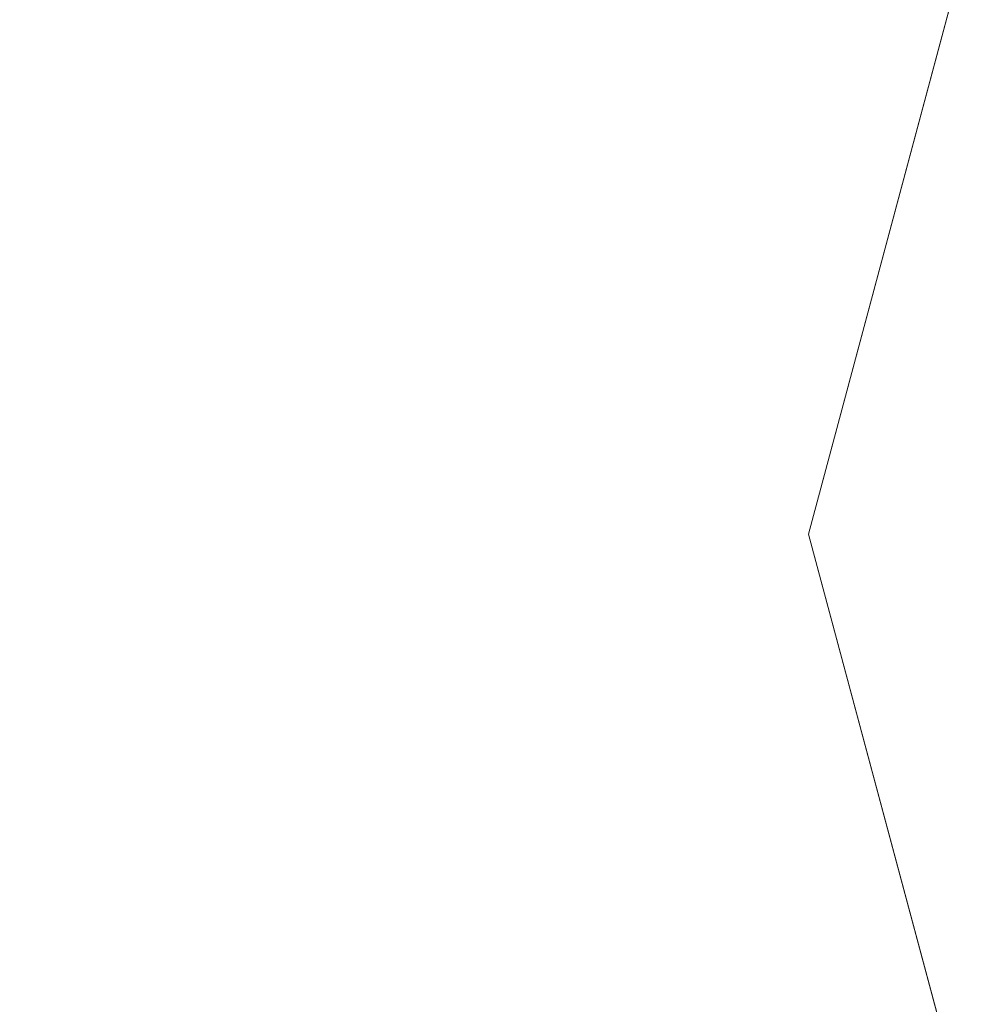
# Model space of a CAD drawing. Units: inches. Extents: x 375 to 1122, y 27 to 1069.
# Tile 107 of 155: x 731.282 to 734.892, y 867.512 to 871.191. Entities that reach past the tile are written whole.
import ezdxf

# ---------------------------------------------------------------- set-up
doc = ezdxf.new("R2010")
doc.units = ezdxf.units.IN
doc.layers.add('A-ANNO-DIMS', color=2, linetype='Continuous', lineweight=18)
doc.layers.add('Furniture', color=30, linetype='Continuous', lineweight=18)
doc.styles.get("Standard").update_dxf_attribs({"font": 'arial.ttf'})
doc.dimstyles.new('ISO-25', dxfattribs={"dimtxt": 12, "dimasz": 2.5, "dimexe": 1.5, "dimexo": 1.5, "dimtad": 1, "dimdec": 1, "dimlunit": 3, "dimtxsty": 'Standard', "dimblk": 'ARCHTICK', "dimcen": 2.5, "dimadec": 0, "dimazin": 0, "dimtfac": 1, "dimtdec": 1, "dimtmove": 0, "dimatfit": 3, "dimfxl": 1.5, "dimfxlon": 1, "dimarcsym": 0})

# ---------------------------------------------------------------- blocks, each defined once
blk = doc.blocks.new('A$C403C54AD')
at = {"linetype": 'ByBlock', "invisible_edges": 5}
for points in [[(1.674179, 1.280047, -0.037345), (1.657248, 1.250721, -0.02811), (1.726512, 1.232162, -0.02811), (1.726512, 1.266024, -0.037345)], [(1.726512, 1.266024, -0.037345), (1.726512, 1.232162, -0.02811), (1.795775, 1.250721, -0.02811), (1.778844, 1.280047, -0.037345)], [(1.657248, 1.250721, -0.023492), (1.666483, 1.266717, -0.023492), (1.726512, 1.250632, -0.023492), (1.726512, 1.232162, -0.023492)], [(1.726512, 1.232162, -0.023492), (1.726512, 1.250632, -0.023492), (1.78654, 1.266717, -0.023492), (1.795775, 1.250721, -0.023492)]]:
    blk.add_3dface(points, dxfattribs=at)
at = {"linetype": 'ByBlock'}
for points in [[(1.657248, 1.250721, -0.02811), (1.657248, 1.250721, -0.023492), (1.726512, 1.232162, -0.023492), (1.726512, 1.232162, -0.02811)], [(1.726512, 1.232162, -0.02811), (1.726512, 1.232162, -0.023492), (1.795775, 1.250721, -0.023492), (1.795775, 1.250721, -0.02811)]]:
    blk.add_3dface(points, dxfattribs=at)
blk = doc.blocks.new('_ArchTick')
at = {"color": 0, "linetype": 'ByBlock', "const_width": 0.15}
blk.add_lwpolyline([(-0.5, -0.5), (0.5, 0.5)], dxfattribs=at)
blk = doc.blocks.new('*D85')
at = {"layer": 'A-ANNO-DIMS', "color": 0, "lineweight": -2, "transparency": 16777216}
for p, q in [((401.5073, 868.5277), (398.5073, 868.5277)), ((400.0073, 814.5277), (400.0073, 868.5277)), ((401.5073, 814.5277), (398.5073, 814.5277))]:
    blk.add_line(p, q, dxfattribs=at)
at = {"layer": 'Defpoints', "color": 0, "transparency": 16777216}
for p in [(400.0073, 868.5277), (845.0073, 868.5277), (845.0073, 814.5277)]:
    blk.add_point(p, dxfattribs=at)
at = {"layer": 'A-ANNO-DIMS', "color": 0, "lineweight": -2, "transparency": 16777216, "xscale": 2.5, "yscale": 2.5, "zscale": 2.5}
for p, rotation in [((400.0073, 868.5277), 90), ((400.0073, 814.5277), 270)]:
    blk.add_blockref('_ArchTick', p, dxfattribs=dict(at, rotation=rotation))
at = {"layer": 'A-ANNO-DIMS', "color": 0, "transparency": 16777216, "insert": (393.2555, 841.5277), "char_height": 12, "attachment_point": 5, "rotation": 90}
blk.add_mtext('4\'-6"', dxfattribs=at)
blk = doc.blocks.new('*D88')
at = {"layer": 'A-ANNO-DIMS', "color": 0, "lineweight": -2, "transparency": 16777216}
for p, q in [((731.0073, 1052.5277), (731.0073, 1055.5277)), ((854.0073, 1052.5277), (854.0073, 1055.5277)), ((731.0073, 1054.0277), (854.0073, 1054.0277))]:
    blk.add_line(p, q, dxfattribs=at)
at = {"layer": 'Defpoints', "color": 0, "transparency": 16777216}
for p in [(854.0073, 1054.0277), (731.0073, 502.5277), (854.0073, 502.5277)]:
    blk.add_point(p, dxfattribs=at)
at = {"layer": 'A-ANNO-DIMS', "color": 0, "lineweight": -2, "transparency": 16777216, "xscale": 2.5, "yscale": 2.5, "zscale": 2.5, "rotation": 180}
blk.add_blockref('_ArchTick', (731.0073, 1054.0277), dxfattribs=at)
at = {"layer": 'A-ANNO-DIMS', "color": 0, "lineweight": -2, "transparency": 16777216, "xscale": 2.5, "yscale": 2.5, "zscale": 2.5}
blk.add_blockref('_ArchTick', (854.0073, 1054.0277), dxfattribs=at)
at = {"layer": 'A-ANNO-DIMS', "color": 0, "transparency": 16777216, "insert": (792.5073, 1060.7837), "char_height": 12, "attachment_point": 5}
blk.add_mtext('10\'-3"', dxfattribs=at)
blk = doc.blocks.new('*D91')
at = {"layer": 'A-ANNO-DIMS', "color": 0, "lineweight": -2, "transparency": 16777216}
for p, q in [((728.0073, 1052.5277), (728.0073, 1055.5277)), ((788.0073, 1052.5277), (788.0073, 1055.5277)), ((728.0073, 1054.0277), (788.0073, 1054.0277))]:
    blk.add_line(p, q, dxfattribs=at)
at = {"layer": 'Defpoints', "color": 0, "transparency": 16777216}
for p in [(788.0073, 1054.0277), (728.0073, 774.0277), (788.0073, 774.0277)]:
    blk.add_point(p, dxfattribs=at)
at = {"layer": 'A-ANNO-DIMS', "color": 0, "lineweight": -2, "transparency": 16777216, "xscale": 2.5, "yscale": 2.5, "zscale": 2.5, "rotation": 180}
blk.add_blockref('_ArchTick', (728.0073, 1054.0277), dxfattribs=at)
at = {"layer": 'A-ANNO-DIMS', "color": 0, "lineweight": -2, "transparency": 16777216, "xscale": 2.5, "yscale": 2.5, "zscale": 2.5}
blk.add_blockref('_ArchTick', (788.0073, 1054.0277), dxfattribs=at)
at = {"layer": 'A-ANNO-DIMS', "color": 0, "transparency": 16777216, "insert": (758.0073, 1060.7796), "char_height": 12, "attachment_point": 5}
blk.add_mtext('5\'-0"', dxfattribs=at)

msp = doc.modelspace()

# ---------------------------------------------------------------- block references
at = {"layer": 'Furniture', "xscale": 39.9918517141215, "yscale": 39.9918517141215, "zscale": 39.9918517141215, "rotation": 270}
msp.add_blockref('A$C403C54AD', (684.9549, 938.3156, 0.024), dxfattribs=at)

# ---------------------------------------------------------------- dimensions: what is measured, and where the dimension line sits
at = {"layer": 'A-ANNO-DIMS'}
for base, p1, p2, picture, middle in [((788.0073, 1054.0277), (728.0073, 774.0277), (788.0073, 774.0277), '*D91', (758.0073, 1060.7796)), ((854.0073, 1054.0277), (731.0073, 502.5277), (854.0073, 502.5277), '*D88', (792.5073, 1060.7837))]:
    dim = msp.add_linear_dim(base=base, p1=p1, p2=p2, dimstyle='ISO-25', override={"dimdec": 1, "dimlfac": 1, "dimrnd": 0, "dimzin": 1, "dimdsep": 46, "dimlunit": 4, "dimfrac": 2}, dxfattribs=at)
    dim.commit()
    dim.dimension.update_dxf_attribs({"geometry": picture, "text_midpoint": middle})
dim = msp.add_linear_dim(base=(400.0073, 868.5277), p1=(845.0073, 814.5277), p2=(845.0073, 868.5277), angle=90, dimstyle='ISO-25', override={"dimdec": 1, "dimlfac": 1, "dimrnd": 0, "dimzin": 1, "dimdsep": 46, "dimlunit": 4, "dimfrac": 2}, dxfattribs=at)
dim.commit()
dim.dimension.update_dxf_attribs({"geometry": '*D85', "text_midpoint": (393.2555, 841.5277)})

doc.saveas('drawing.dxf')
